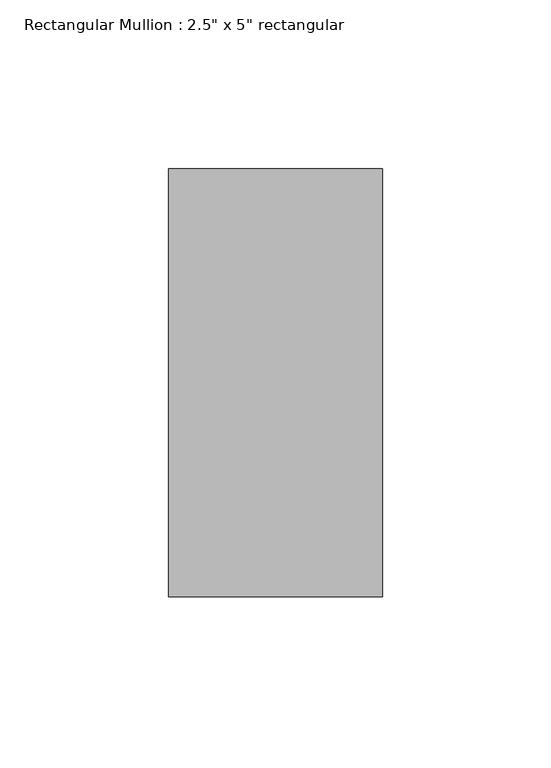
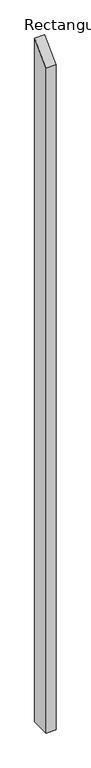
"""IFC4 building model written with IfcOpenShell, lengths in millimetres: member geometry."""

from ifc_helpers import new_model, si_unit, frame, origin, place, context, project, spatial, polyline, outline, extrude, source, transform, mapped, element, save


def member_2fad0b47(model_context):
    return source(origin(), model_context, "Body", "SweptSolid", [
        extrude(outline(polyline([(-63.5, -63.5), (63.5, 63.5), (63.5, -4576.0368176), (-63.5, -4576.0368176), (-63.5, -63.5)])), frame((-63.5, 0.0, 0.0), z_axis=(1.0, 0.0, 0.0), x_axis=(0.0, 1.0, 0.0)), (0.0, 0.0, 1.0), 63.5),
    ])


if __name__ == "__main__":
    model = new_model("IFC4")
    model_context = context("Model", 3, world=origin())
    ifc_project = project(units=[si_unit("LENGTHUNIT", "METRE", prefix="MILLI")], contexts=[model_context])
    site = spatial("IfcSite", under=ifc_project)
    building = spatial("IfcBuilding", under=site)
    placement = place(None, origin())
    member_shape = member_2fad0b47(model_context)
    element("IfcMember", 1, ObjectType="Rectangular Mullion : 2.5\" x 5\" rectangular", at=placement, inside=building, context=model_context, shape_type="MappedRepresentation", body=[
        mapped(member_shape, transform((0.0, 0.0, 0.0), x_axis=(1.0, 0.0, 0.0), y_axis=(0.0, 1.0, 0.0), z_axis=(0.0, 0.0, 1.0))),
    ])
    save(model, "model.ifc")

# Revit data of these elements
# Type "Rectangular Mullion : 2.5\" x 5\" rectangular"
#   built-in parameter 1007304 = 0.416667 (stored number, unit not read)
#   built-in parameter 1007301 = 0.104167 (stored number, unit not read)
#   built-in parameter 1007300 = 0.104167 (stored number, unit not read)
# Element 1 (IfcMember, "Rectangular Mullion : 2.5\" x 5\" rectangular")
#   Materials on its faces: "Aluminum"
# Materials
#   "Aluminum": class "Metal", colour RGB 247 247 247, transparency 0, Description = "Aluminum 6061", Cost = 0
